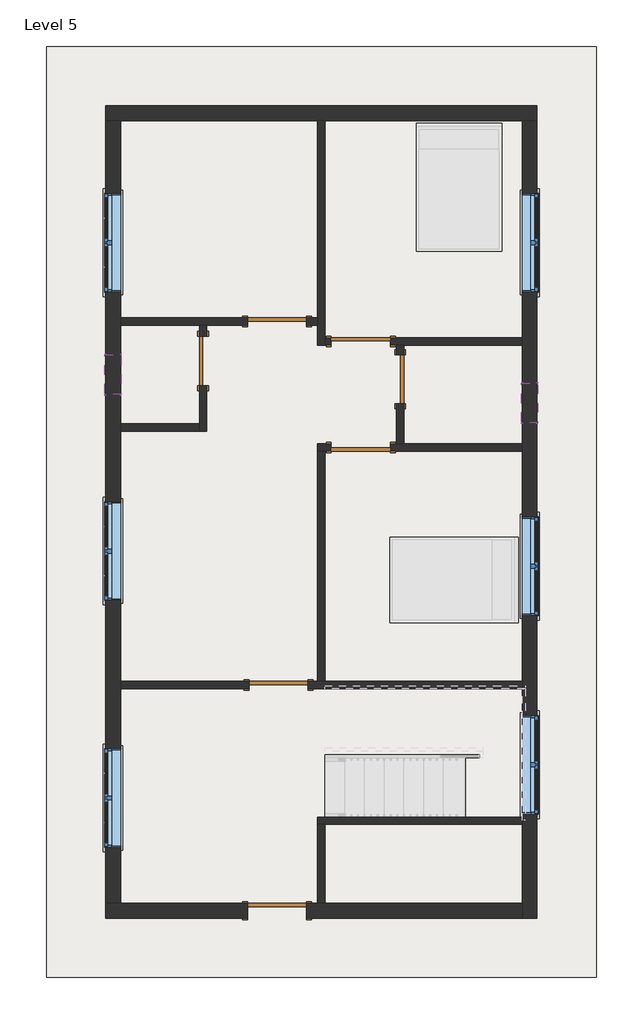
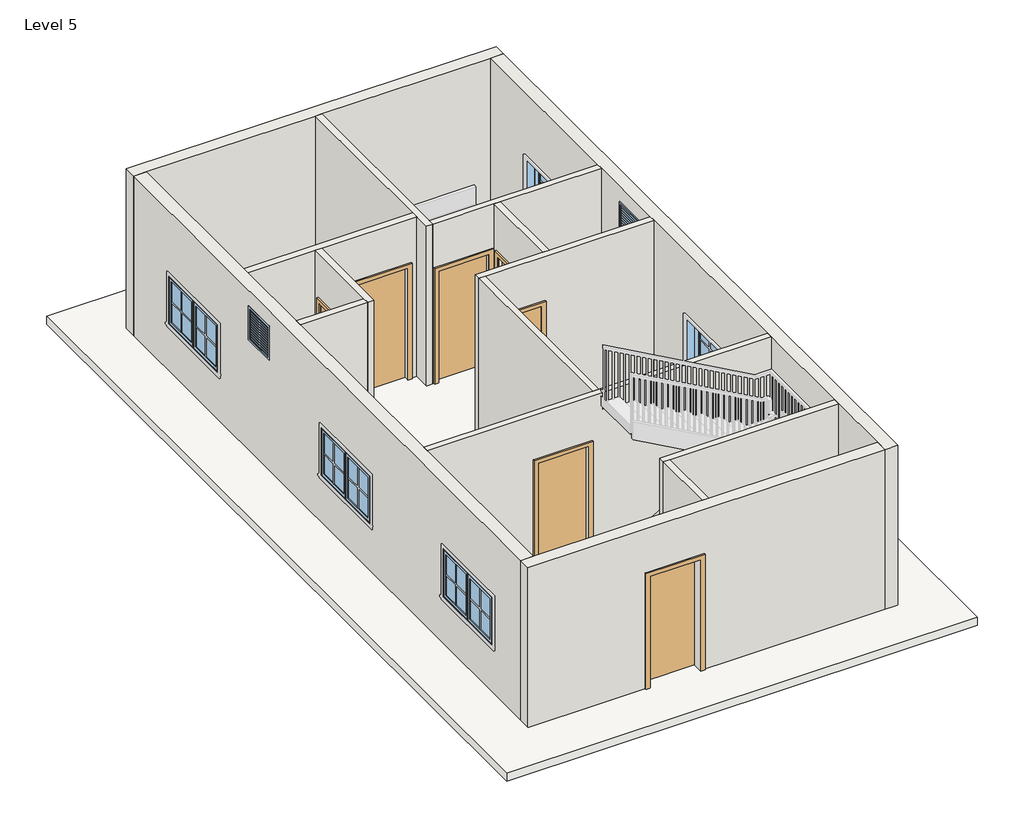
# One storey, part 1 of 3: 15 walls, 8 windows, 7 doors, 1 roof.
"""IFC4 building model written with IfcOpenShell, lengths in millimetres."""

from ifc_helpers import new_model, si_unit, frame, origin, place, context, project, spatial, polyline, outline, extrude, faceted_brep, transform, mapped, element, save
from components import door_78caadf7, door_214872d5, single_flush_door_3_e5f9f3c4, single_flush_door_3_305aa2a5, single_flush_door_3_0ca8825f, window_casement_double_win_5_c1d95f0f, window_f2d8fef0

model = new_model("IFC4")

# Units and contexts
model_context = context("Model", 3, world=origin())
ifc_project = project(units=[si_unit("LENGTHUNIT", "METRE", prefix="MILLI")], contexts=[model_context])

# Site, building, storey
site = spatial("IfcSite", under=ifc_project)
building = spatial("IfcBuilding", under=site)
storey = spatial("IfcBuildingStorey", under=building, Name="Level 5", Elevation=12649.2)

# Doors
placement = place(None, origin())
door_shape = door_78caadf7(model_context)
element("IfcDoor", 1, ObjectType="Single-Flush : 2'6\"", at=placement, inside=storey, context=model_context, shape_type="MappedRepresentation", body=[
    mapped(door_shape, transform((-35.92188, 1946.24131, 12649.2), x_axis=(0.0, 1.0, 0.0), y_axis=(-1.0, 0.0, 0.0), z_axis=(0.0, 0.0, 1.0))),
])
door_2_shape = door_214872d5(model_context)
element("IfcDoor", 2, ObjectType="Single-Flush : 2'6\"", at=placement, inside=storey, context=model_context, shape_type="MappedRepresentation", body=[
    mapped(door_2_shape, transform((-3083.92188, 2225.64131, 12649.2), x_axis=(0.0, 1.0, 0.0), y_axis=(-1.0, 0.0, 0.0), z_axis=(0.0, 0.0, 1.0))),
])
single_flush_door_3_shape = single_flush_door_3_e5f9f3c4(model_context)
element("IfcDoor", 3, ObjectType="Single-Flush : DOOR 3'", at=placement, inside=storey, context=model_context, shape_type="MappedRepresentation", body=[
    mapped(single_flush_door_3_shape, transform((-1940.92188, 2835.24131, 12649.2), x_axis=(1.0, 0.0, 0.0), y_axis=(0.0, 1.0, 0.0), z_axis=(0.0, 0.0, 1.0))),
])
element("IfcDoor", 4, ObjectType="Single-Flush : DOOR 3'", at=placement, inside=storey, context=model_context, shape_type="MappedRepresentation", body=[
    mapped(single_flush_door_3_shape, transform((-645.52188, 892.14131, 12649.2), x_axis=(-1.0, 0.0, 0.0), y_axis=(0.0, -1.0, 0.0), z_axis=(0.0, 0.0, 1.0))),
])
element("IfcDoor", 5, ObjectType="Single-Flush : DOOR 3'", at=placement, inside=storey, context=model_context, shape_type="MappedRepresentation", body=[
    mapped(single_flush_door_3_shape, transform((-1915.52188, -2778.15869, 12649.2), x_axis=(1.0, 0.0, 0.0), y_axis=(0.0, 1.0, 0.0), z_axis=(0.0, 0.0, 1.0))),
])
single_flush_door_3_2_shape = single_flush_door_3_305aa2a5(model_context)
element("IfcDoor", 6, ObjectType="Single-Flush : DOOR 3'", at=placement, inside=storey, context=model_context, shape_type="MappedRepresentation", body=[
    mapped(single_flush_door_3_2_shape, transform((-645.52188, 2530.44131, 12649.2), x_axis=(-1.0, 0.0, 0.0), y_axis=(0.0, -1.0, 0.0), z_axis=(0.0, 0.0, 1.0))),
])
single_flush_door_3_3_shape = single_flush_door_3_0ca8825f(model_context)
element("IfcDoor", 7, ObjectType="Single-Flush : DOOR 3'", at=placement, inside=storey, context=model_context, shape_type="MappedRepresentation", body=[
    mapped(single_flush_door_3_3_shape, transform((-1940.92188, -6264.30869, 12649.2), x_axis=(1.0, 0.0, 0.0), y_axis=(0.0, 1.0, 0.0), z_axis=(0.0, 0.0, 1.0))),
])

# Roof
element("IfcRoof", 8, ObjectType="ROOF 6\"", at=placement, inside=storey, context=model_context, shape_type="SweptSolid", body=[
    extrude(outline(polyline([(-5503.27188, 7083.39131), (2993.02812, 7083.39131), (2993.02812, -7293.00869), (-5503.27188, -7293.00869), (-5503.27188, 7083.39131)])), frame((0.0, 0.0, 12496.8), z_axis=(0.0, 0.0, 1.0), x_axis=(1.0, 0.0, 0.0)), (0.0, 0.0, 1.0), 152.4),
])

# Walls
element("IfcWall", 9, ObjectType="WALL 4.5'", at=placement, inside=storey, context=model_context, shape_type="Brep", body=[
    faceted_brep([(-1312.27188, 5940.39131, 12649.2), (-1312.27188, 2892.39131, 12649.2), (-1312.27188, 2778.09131, 12649.2), (-1312.27188, 2473.29131, 12649.2), (-1312.27188, 2473.29131, 15697.2), (-1312.27188, 2778.09131, 15697.2), (-1312.27188, 2892.39131, 15697.2), (-1312.27188, 5940.39131, 15697.2), (-1197.97188, 5940.39131, 12649.2), (-1197.97188, 5940.39131, 15697.2), (-1197.97188, 2587.59131, 15697.2), (-1197.97188, 2473.29131, 15697.2), (-1197.97188, 2473.29131, 12649.2), (-1197.97188, 2587.59131, 12649.2)], [[[0, 1, 2, 3, 4, 5, 6, 7]], [[8, 9, 10, 11, 12, 13]], [[3, 2, 1, 0, 8, 13, 12]], [[0, 7, 9, 8]], [[4, 3, 12, 11]], [[7, 6, 5, 4, 11, 10, 9]]]),
])
element("IfcWall", 10, ObjectType="WALL 4.5'", at=placement, inside=storey, context=model_context, shape_type="Brep", body=[
    faceted_brep([(-1197.97188, 2473.29131, 12649.2), (-1102.72188, 2473.29131, 12649.2), (-1102.72188, 2473.29131, 14782.8), (-188.32188, 2473.29131, 14782.8), (-188.32188, 2473.29131, 12649.2), (-93.07188, 2473.29131, 12649.2), (21.22812, 2473.29131, 12649.2), (1850.02812, 2473.29131, 12649.2), (1850.02812, 2473.29131, 15697.2), (21.22812, 2473.29131, 15697.2), (-93.07188, 2473.29131, 15697.2), (-1197.97188, 2473.29131, 15697.2), (-1102.72188, 2587.59131, 14782.8), (-1102.72188, 2587.59131, 12649.2), (-1197.97188, 2587.59131, 12649.2), (-1197.97188, 2587.59131, 15697.2), (1850.02812, 2587.59131, 15697.2), (1850.02812, 2587.59131, 12649.2), (-188.32188, 2587.59131, 12649.2), (-188.32188, 2587.59131, 14782.8)], [[[0, 1, 2, 3, 4, 5, 6, 7, 8, 9, 10, 11]], [[12, 13, 14, 15, 16, 17, 18, 19]], [[18, 17, 7, 6, 5, 4]], [[14, 13, 1, 0]], [[0, 11, 15, 14]], [[8, 7, 17, 16]], [[2, 1, 13, 12]], [[3, 2, 12, 19]], [[4, 3, 19, 18]], [[11, 10, 9, 8, 16, 15]]]),
])
element("IfcWall", 11, ObjectType="WALL 4.5'", at=placement, inside=storey, context=model_context, shape_type="Brep", body=[
    faceted_brep([(-1312.27188, 2892.39131, 12649.2), (-1483.72188, 2892.39131, 12649.2), (-1483.72188, 2892.39131, 14782.8), (-2398.12188, 2892.39131, 14782.8), (-2398.12188, 2892.39131, 12649.2), (-4360.27188, 2892.39131, 12649.2), (-4360.27188, 2892.39131, 15697.2), (-1312.27188, 2892.39131, 15697.2), (-1483.72188, 2778.09131, 14782.8), (-1483.72188, 2778.09131, 12649.2), (-1312.27188, 2778.09131, 12649.2), (-1312.27188, 2778.09131, 15697.2), (-3026.77188, 2778.09131, 15697.2), (-3141.07188, 2778.09131, 15697.2), (-4360.27188, 2778.09131, 15697.2), (-4360.27188, 2778.09131, 12649.2), (-3141.07188, 2778.09131, 12649.2), (-3026.77188, 2778.09131, 12649.2), (-2398.12188, 2778.09131, 12649.2), (-2398.12188, 2778.09131, 14782.8)], [[[0, 1, 2, 3, 4, 5, 6, 7]], [[8, 9, 10, 11, 12, 13, 14, 15, 16, 17, 18, 19]], [[10, 9, 1, 0]], [[18, 17, 16, 15, 5, 4]], [[6, 5, 15, 14]], [[0, 7, 11, 10]], [[2, 1, 9, 8]], [[3, 2, 8, 19]], [[4, 3, 19, 18]], [[7, 6, 14, 13, 12, 11]]]),
])
element("IfcWall", 12, ObjectType="WALL 4.5'", at=placement, inside=storey, context=model_context, shape_type="Brep", body=[
    faceted_brep([(-3141.07188, 2778.09131, 12649.2), (-3141.07188, 2606.64131, 12649.2), (-3141.07188, 2606.64131, 14782.8), (-3141.07188, 1844.64131, 14782.8), (-3141.07188, 1844.64131, 12649.2), (-3141.07188, 1254.09131, 12649.2), (-3141.07188, 1139.79131, 12649.2), (-3141.07188, 1139.79131, 15697.2), (-3141.07188, 1254.09131, 15697.2), (-3141.07188, 2778.09131, 15697.2), (-3026.77188, 2606.64131, 14782.8), (-3026.77188, 2606.64131, 12649.2), (-3026.77188, 2778.09131, 12649.2), (-3026.77188, 2778.09131, 15697.2), (-3026.77188, 1139.79131, 15697.2), (-3026.77188, 1139.79131, 12649.2), (-3026.77188, 1844.64131, 12649.2), (-3026.77188, 1844.64131, 14782.8)], [[[0, 1, 2, 3, 4, 5, 6, 7, 8, 9]], [[10, 11, 12, 13, 14, 15, 16, 17]], [[16, 15, 6, 5, 4]], [[12, 11, 1, 0]], [[0, 9, 13, 12]], [[7, 6, 15, 14]], [[2, 1, 11, 10]], [[3, 2, 10, 17]], [[4, 3, 17, 16]], [[9, 8, 7, 14, 13]]]),
])
element("IfcWall", 13, ObjectType="WALL 4.5'", at=placement, inside=storey, context=model_context, shape_type="SweptSolid", body=[
    extrude(outline(polyline([(-4360.27188, 1254.09131), (-3141.07188, 1254.09131), (-3141.07188, 1139.79131), (-4360.27188, 1139.79131), (-4360.27188, 1254.09131)])), frame((0.0, 0.0, 12649.2), z_axis=(0.0, 0.0, 1.0), x_axis=(1.0, 0.0, 0.0)), (0.0, 0.0, 1.0), 3048.0),
])
element("IfcWall", 14, ObjectType="WALL 4.5'", at=placement, inside=storey, context=model_context, shape_type="SweptSolid", body=[
    extrude(outline(polyline([(2473.29131, 12649.2), (2327.24131, 12649.2), (2327.24131, 14782.8), (1565.24131, 14782.8), (1565.24131, 12649.2), (949.29131, 12649.2), (949.29131, 15697.2), (2473.29131, 15697.2), (2473.29131, 12649.2)])), frame((-93.07188, 0.0, 0.0), z_axis=(1.0, 0.0, 0.0), x_axis=(0.0, 1.0, 0.0)), (0.0, 0.0, 1.0), 114.3),
])
element("IfcWall", 15, ObjectType="WALL 4.5'", at=placement, inside=storey, context=model_context, shape_type="Brep", body=[
    faceted_brep([(-1102.72188, 949.29131, 14782.8), (-1102.72188, 949.29131, 12649.2), (-1312.27188, 949.29131, 12649.2), (-1312.27188, 949.29131, 15697.2), (-93.07188, 949.29131, 15697.2), (21.22812, 949.29131, 15697.2), (1850.02812, 949.29131, 15697.2), (1850.02812, 949.29131, 12649.2), (21.22812, 949.29131, 12649.2), (-93.07188, 949.29131, 12649.2), (-188.32188, 949.29131, 12649.2), (-188.32188, 949.29131, 14782.8), (-1312.27188, 834.99131, 12649.2), (-1197.97188, 834.99131, 12649.2), (-1102.72188, 834.99131, 12649.2), (-1102.72188, 834.99131, 14782.8), (-188.32188, 834.99131, 14782.8), (-188.32188, 834.99131, 12649.2), (1850.02812, 834.99131, 12649.2), (1850.02812, 834.99131, 15697.2), (-1197.97188, 834.99131, 15697.2), (-1312.27188, 834.99131, 15697.2)], [[[0, 1, 2, 3, 4, 5, 6, 7, 8, 9, 10, 11]], [[12, 13, 14, 15, 16, 17, 18, 19, 20, 21]], [[2, 1, 14, 13, 12]], [[10, 9, 8, 7, 18, 17]], [[7, 6, 19, 18]], [[3, 2, 12, 21]], [[15, 14, 1, 0]], [[16, 15, 0, 11]], [[17, 16, 11, 10]], [[6, 5, 4, 3, 21, 20, 19]]]),
])
element("IfcWall", 16, ObjectType="WALL 4.5'", at=placement, inside=storey, context=model_context, shape_type="SweptSolid", body=[
    extrude(outline(polyline([(-1312.27188, -2721.00869), (-1312.27188, 834.99131), (-1197.97188, 834.99131), (-1197.97188, -2721.00869), (-1312.27188, -2721.00869)])), frame((0.0, 0.0, 12649.2), z_axis=(0.0, 0.0, 1.0), x_axis=(1.0, 0.0, 0.0)), (0.0, 0.0, 1.0), 3048.0),
])
element("IfcWall", 17, ObjectType="WALL 4.5'", at=placement, inside=storey, context=model_context, shape_type="Brep", body=[
    faceted_brep([(1850.02812, -2721.00869, 12649.2), (-1197.97188, -2721.00869, 12649.2), (-1312.27188, -2721.00869, 12649.2), (-1458.32188, -2721.00869, 12649.2), (-1458.32188, -2721.00869, 14782.8), (-2372.72188, -2721.00869, 14782.8), (-2372.72188, -2721.00869, 12649.2), (-4360.27188, -2721.00869, 12649.2), (-4360.27188, -2721.00869, 15697.2), (-1312.27188, -2721.00869, 15697.2), (-1197.97188, -2721.00869, 15697.2), (1850.02812, -2721.00869, 15697.2), (-1458.32188, -2835.30869, 14782.8), (-1458.32188, -2835.30869, 12649.2), (1850.02812, -2835.30869, 12649.2), (1850.02812, -2835.30869, 15697.2), (-4360.27188, -2835.30869, 15697.2), (-4360.27188, -2835.30869, 12649.2), (-2372.72188, -2835.30869, 12649.2), (-2372.72188, -2835.30869, 14782.8)], [[[0, 1, 2, 3, 4, 5, 6, 7, 8, 9, 10, 11]], [[12, 13, 14, 15, 16, 17, 18, 19]], [[18, 17, 7, 6]], [[14, 13, 3, 2, 1, 0]], [[0, 11, 15, 14]], [[8, 7, 17, 16]], [[4, 3, 13, 12]], [[5, 4, 12, 19]], [[6, 5, 19, 18]], [[11, 10, 9, 8, 16, 15]]]),
])
element("IfcWall", 18, ObjectType="WALL 4.5'", at=placement, inside=storey, context=model_context, shape_type="Brep", body=[
    faceted_brep([(1850.02812, -4816.50869, 12649.2), (-1312.27188, -4816.50869, 12649.2), (-1312.27188, -4816.50869, 15697.2), (1850.02812, -4816.50869, 15697.2), (1850.02812, -4930.80869, 12649.2), (1850.02812, -4930.80869, 15697.2), (-1197.97188, -4930.80869, 15697.2), (-1312.27188, -4930.80869, 15697.2), (-1312.27188, -4930.80869, 12649.2), (-1197.97188, -4930.80869, 12649.2)], [[[0, 1, 2, 3]], [[4, 5, 6, 7, 8, 9]], [[1, 0, 4, 9, 8]], [[0, 3, 5, 4]], [[2, 1, 8, 7]], [[3, 2, 7, 6, 5]]]),
])
element("IfcWall", 19, ObjectType="WALL 4.5'", at=placement, inside=storey, context=model_context, shape_type="SweptSolid", body=[
    extrude(outline(polyline([(-1312.27188, -6150.00869), (-1312.27188, -4930.80869), (-1197.97188, -4930.80869), (-1197.97188, -6150.00869), (-1312.27188, -6150.00869)])), frame((0.0, 0.0, 12649.2), z_axis=(0.0, 0.0, 1.0), x_axis=(1.0, 0.0, 0.0)), (0.0, 0.0, 1.0), 3048.0),
])
element("IfcWall", 20, ObjectType="WALL 9\"", at=placement, inside=storey, context=model_context, shape_type="Brep", body=[
    faceted_brep([(-4588.87188, 5940.39131, 12649.2), (-4360.27188, 5940.39131, 12649.2), (-1312.27188, 5940.39131, 12649.2), (-1197.97188, 5940.39131, 12649.2), (1850.02812, 5940.39131, 12649.2), (2078.62812, 5940.39131, 12649.2), (2078.62812, 5940.39131, 15697.2), (1850.02812, 5940.39131, 15697.2), (-1197.97188, 5940.39131, 15697.2), (-1312.27188, 5940.39131, 15697.2), (-4360.27188, 5940.39131, 15697.2), (-4588.87188, 5940.39131, 15697.2), (-4588.87188, 6168.99131, 12649.2), (-4588.87188, 6168.99131, 15697.2), (2078.62812, 6168.99131, 15697.2), (2078.62812, 6168.99131, 12649.2)], [[[0, 1, 2, 3, 4, 5, 6, 7, 8, 9, 10, 11]], [[12, 13, 14, 15]], [[5, 4, 3, 2, 1, 0, 12, 15]], [[6, 5, 15, 14]], [[0, 11, 13, 12]], [[11, 10, 9, 8, 7, 6, 14, 13]]]),
])
element("IfcWall", 21, ObjectType="WALL 9\"", at=placement, inside=storey, context=model_context, shape_type="Brep", body=[
    faceted_brep([(1850.02812, 5940.39131, 12649.2), (1850.02812, 2587.59131, 12649.2), (1850.02812, 2473.29131, 12649.2), (1850.02812, 949.29131, 12649.2), (1850.02812, 834.99131, 12649.2), (1850.02812, -2721.00869, 12649.2), (1850.02812, -2835.30869, 12649.2), (1850.02812, -4816.50869, 12649.2), (1850.02812, -4930.80869, 12649.2), (1850.02812, -6150.00869, 12649.2), (1850.02812, -6378.60869, 12649.2), (1850.02812, -6378.60869, 15697.2), (1850.02812, -6150.00869, 15697.2), (1850.02812, -4930.80869, 15697.2), (1850.02812, -4816.50869, 15697.2), (1850.02812, -2835.30869, 15697.2), (1850.02812, -2721.00869, 15697.2), (1850.02812, 834.99131, 15697.2), (1850.02812, 949.29131, 15697.2), (1850.02812, 2473.29131, 15697.2), (1850.02812, 2587.59131, 15697.2), (1850.02812, 5940.39131, 15697.2), (1850.02812, -4772.05869, 14478.0), (1850.02812, -4772.05869, 13563.6), (1850.02812, -3248.05869, 13563.6), (1850.02812, -3248.05869, 14478.0), (1850.02812, 3292.44131, 14478.0), (1850.02812, 3292.44131, 13563.6), (1850.02812, 4816.44131, 13563.6), (1850.02812, 4816.44131, 14478.0), (1850.02812, -1705.00869, 14478.0), (1850.02812, -1705.00869, 13563.6), (1850.02812, -181.00869, 13563.6), (1850.02812, -181.00869, 14478.0), (1850.02812, 1273.14131, 15392.4), (1850.02812, 1273.14131, 14782.8), (1850.02812, 1882.74131, 14782.8), (1850.02812, 1882.74131, 15392.4), (2078.62812, 5940.39131, 12649.2), (2078.62812, 5940.39131, 15697.2), (2078.62812, -6378.60869, 15697.2), (2078.62812, -6378.60869, 12649.2), (2078.62812, -4772.05869, 14478.0), (2078.62812, -3248.05869, 14478.0), (2078.62812, -3248.05869, 13563.6), (2078.62812, -4772.05869, 13563.6), (2078.62812, 3292.44131, 14478.0), (2078.62812, 4816.44131, 14478.0), (2078.62812, 4816.44131, 13563.6), (2078.62812, 3292.44131, 13563.6), (2078.62812, -1705.00869, 14478.0), (2078.62812, -181.00869, 14478.0), (2078.62812, -181.00869, 13563.6), (2078.62812, -1705.00869, 13563.6), (2078.62812, 1273.14131, 15392.4), (2078.62812, 1882.74131, 15392.4), (2078.62812, 1882.74131, 14782.8), (2078.62812, 1273.14131, 14782.8)], [[[0, 1, 2, 3, 4, 5, 6, 7, 8, 9, 10, 11, 12, 13, 14, 15, 16, 17, 18, 19, 20, 21], [22, 23, 24, 25], [26, 27, 28, 29], [30, 31, 32, 33], [34, 35, 36, 37]], [[38, 39, 40, 41], [42, 43, 44, 45], [46, 47, 48, 49], [50, 51, 52, 53], [54, 55, 56, 57]], [[10, 9, 8, 7, 6, 5, 4, 3, 2, 1, 0, 38, 41]], [[0, 21, 39, 38]], [[11, 10, 41, 40]], [[23, 22, 42, 45]], [[24, 23, 45, 44]], [[25, 24, 44, 43]], [[22, 25, 43, 42]], [[27, 26, 46, 49]], [[28, 27, 49, 48]], [[29, 28, 48, 47]], [[26, 29, 47, 46]], [[31, 30, 50, 53]], [[32, 31, 53, 52]], [[33, 32, 52, 51]], [[30, 33, 51, 50]], [[35, 34, 54, 57]], [[36, 35, 57, 56]], [[37, 36, 56, 55]], [[34, 37, 55, 54]], [[21, 20, 19, 18, 17, 16, 15, 14, 13, 12, 11, 40, 39]]]),
])
element("IfcWall", 22, ObjectType="WALL 9\"", at=placement, inside=storey, context=model_context, shape_type="Brep", body=[
    faceted_brep([(1850.02812, -6150.00869, 12649.2), (-1197.97188, -6150.00869, 12649.2), (-1312.27188, -6150.00869, 12649.2), (-1483.72188, -6150.00869, 12649.2), (-1483.72188, -6150.00869, 14782.8), (-2398.12188, -6150.00869, 14782.8), (-2398.12188, -6150.00869, 12649.2), (-4360.27188, -6150.00869, 12649.2), (-4588.87188, -6150.00869, 12649.2), (-4588.87188, -6150.00869, 15697.2), (-4360.27188, -6150.00869, 15697.2), (-1312.27188, -6150.00869, 15697.2), (-1197.97188, -6150.00869, 15697.2), (1850.02812, -6150.00869, 15697.2), (-1483.72188, -6378.60869, 14782.8), (-1483.72188, -6378.60869, 12649.2), (1850.02812, -6378.60869, 12649.2), (1850.02812, -6378.60869, 15697.2), (-4588.87188, -6378.60869, 15697.2), (-4588.87188, -6378.60869, 12649.2), (-2398.12188, -6378.60869, 12649.2), (-2398.12188, -6378.60869, 14782.8)], [[[0, 1, 2, 3, 4, 5, 6, 7, 8, 9, 10, 11, 12, 13]], [[14, 15, 16, 17, 18, 19, 20, 21]], [[20, 19, 8, 7, 6]], [[16, 15, 3, 2, 1, 0]], [[0, 13, 17, 16]], [[9, 8, 19, 18]], [[4, 3, 15, 14]], [[5, 4, 14, 21]], [[6, 5, 21, 20]], [[13, 12, 11, 10, 9, 18, 17]]]),
])
element("IfcWall", 23, ObjectType="WALL 9\"", at=placement, inside=storey, context=model_context, shape_type="Brep", body=[
    faceted_brep([(-4360.27188, -6150.00869, 12649.2), (-4360.27188, -2835.30869, 12649.2), (-4360.27188, -2721.00869, 12649.2), (-4360.27188, 1139.79131, 12649.2), (-4360.27188, 1254.09131, 12649.2), (-4360.27188, 2778.09131, 12649.2), (-4360.27188, 2892.39131, 12649.2), (-4360.27188, 5940.39131, 12649.2), (-4360.27188, 5940.39131, 15697.2), (-4360.27188, 2892.39131, 15697.2), (-4360.27188, 2778.09131, 15697.2), (-4360.27188, 1254.09131, 15697.2), (-4360.27188, 1139.79131, 15697.2), (-4360.27188, -2721.00869, 15697.2), (-4360.27188, -2835.30869, 15697.2), (-4360.27188, -6150.00869, 15697.2), (-4360.27188, 4816.44131, 14478.0), (-4360.27188, 4816.44131, 13563.6), (-4360.27188, 3292.44131, 13563.6), (-4360.27188, 3292.44131, 14478.0), (-4360.27188, 53.94131, 14478.0), (-4360.27188, 53.94131, 13563.6), (-4360.27188, -1470.05869, 13563.6), (-4360.27188, -1470.05869, 14478.0), (-4360.27188, -3759.23369, 14478.0), (-4360.27188, -3759.23369, 13563.6), (-4360.27188, -5283.23369, 13563.6), (-4360.27188, -5283.23369, 14478.0), (-4360.27188, 1711.29131, 15392.4), (-4360.27188, 2320.89131, 15392.4), (-4360.27188, 2320.89131, 14782.8), (-4360.27188, 1711.29131, 14782.8), (-4588.87188, -6150.00869, 12649.2), (-4588.87188, -6150.00869, 15697.2), (-4588.87188, 5940.39131, 15697.2), (-4588.87188, 5940.39131, 12649.2), (-4588.87188, 4816.44131, 14478.0), (-4588.87188, 3292.44131, 14478.0), (-4588.87188, 3292.44131, 13563.6), (-4588.87188, 4816.44131, 13563.6), (-4588.87188, 53.94131, 14478.0), (-4588.87188, -1470.05869, 14478.0), (-4588.87188, -1470.05869, 13563.6), (-4588.87188, 53.94131, 13563.6), (-4588.87188, -3759.23369, 14478.0), (-4588.87188, -5283.23369, 14478.0), (-4588.87188, -5283.23369, 13563.6), (-4588.87188, -3759.23369, 13563.6), (-4588.87188, 1711.29131, 15392.4), (-4588.87188, 1711.29131, 14782.8), (-4588.87188, 2320.89131, 14782.8), (-4588.87188, 2320.89131, 15392.4)], [[[0, 1, 2, 3, 4, 5, 6, 7, 8, 9, 10, 11, 12, 13, 14, 15], [16, 17, 18, 19], [20, 21, 22, 23], [24, 25, 26, 27], [28, 29, 30, 31]], [[32, 33, 34, 35], [36, 37, 38, 39], [40, 41, 42, 43], [44, 45, 46, 47], [48, 49, 50, 51]], [[7, 6, 5, 4, 3, 2, 1, 0, 32, 35]], [[8, 7, 35, 34]], [[0, 15, 33, 32]], [[17, 16, 36, 39]], [[18, 17, 39, 38]], [[19, 18, 38, 37]], [[16, 19, 37, 36]], [[21, 20, 40, 43]], [[22, 21, 43, 42]], [[23, 22, 42, 41]], [[20, 23, 41, 40]], [[25, 24, 44, 47]], [[26, 25, 47, 46]], [[27, 26, 46, 45]], [[24, 27, 45, 44]], [[49, 48, 28, 31]], [[50, 49, 31, 30]], [[51, 50, 30, 29]], [[48, 51, 29, 28]], [[15, 14, 13, 12, 11, 10, 9, 8, 34, 33]]]),
])

# Windows
window_casement_double_win_5_shape = window_casement_double_win_5_c1d95f0f(model_context)
element("IfcWindow", 24, ObjectType="Window-Casement-Double : WIN 5'", at=placement, inside=storey, context=model_context, shape_type="MappedRepresentation", body=[
    mapped(window_casement_double_win_5_shape, transform((-4474.57188, 4054.44131, 12649.2), x_axis=(0.0, 1.0, 0.0), y_axis=(-1.0, 0.0, 0.0), z_axis=(0.0, 0.0, 1.0))),
])
element("IfcWindow", 25, ObjectType="Window-Casement-Double : WIN 5'", at=placement, inside=storey, context=model_context, shape_type="MappedRepresentation", body=[
    mapped(window_casement_double_win_5_shape, transform((-4474.57188, -708.05869, 12649.2), x_axis=(0.0, 1.0, 0.0), y_axis=(-1.0, 0.0, 0.0), z_axis=(0.0, 0.0, 1.0))),
])
element("IfcWindow", 26, ObjectType="Window-Casement-Double : WIN 5'", at=placement, inside=storey, context=model_context, shape_type="MappedRepresentation", body=[
    mapped(window_casement_double_win_5_shape, transform((-4474.57188, -4521.23369, 12649.2), x_axis=(0.0, 1.0, 0.0), y_axis=(-1.0, 0.0, 0.0), z_axis=(0.0, 0.0, 1.0))),
])
element("IfcWindow", 27, ObjectType="Window-Casement-Double : WIN 5'", at=placement, inside=storey, context=model_context, shape_type="MappedRepresentation", body=[
    mapped(window_casement_double_win_5_shape, transform((1964.32812, -4010.05869, 12649.2), x_axis=(0.0, -1.0, 0.0), y_axis=(1.0, 0.0, 0.0), z_axis=(0.0, 0.0, 1.0))),
])
element("IfcWindow", 28, ObjectType="Window-Casement-Double : WIN 5'", at=placement, inside=storey, context=model_context, shape_type="MappedRepresentation", body=[
    mapped(window_casement_double_win_5_shape, transform((1964.32812, 4054.44131, 12649.2), x_axis=(0.0, -1.0, 0.0), y_axis=(1.0, 0.0, 0.0), z_axis=(0.0, 0.0, 1.0))),
])
element("IfcWindow", 29, ObjectType="Window-Casement-Double : WIN 5'", at=placement, inside=storey, context=model_context, shape_type="MappedRepresentation", body=[
    mapped(window_casement_double_win_5_shape, transform((1964.32812, -943.00869, 12649.2), x_axis=(0.0, -1.0, 0.0), y_axis=(1.0, 0.0, 0.0), z_axis=(0.0, 0.0, 1.0))),
])
window_shape = window_f2d8fef0(model_context)
element("IfcWindow", 30, ObjectType="Window-Louvers : 24\" x 24\"", at=placement, inside=storey, context=model_context, shape_type="MappedRepresentation", body=[
    mapped(window_shape, transform((1957.97812, 1577.94131, 13868.4), x_axis=(0.0, 1.0, 0.0), y_axis=(-1.0, 0.0, 0.0), z_axis=(0.0, 0.0, 1.0))),
])
element("IfcWindow", 31, ObjectType="Window-Louvers : 24\" x 24\"", at=placement, inside=storey, context=model_context, shape_type="MappedRepresentation", body=[
    mapped(window_shape, transform((-4480.92188, 2016.09131, 13868.4), x_axis=(0.0, 1.0, 0.0), y_axis=(-1.0, 0.0, 0.0), z_axis=(0.0, 0.0, 1.0))),
])

save(model, "model.ifc")

# Revit data of these elements
# Type "Single-Flush : 2'6\""
#   Type Mark = "9"
#   Construction Type Id = "MDOOR"
#   Assembly Code = "C1020"
#   Analytic Construction = "Metal"
#   Thickness = 0' - 2"
#   Heat Transfer Coefficient (U) = 0.651978 BTU/(h·ft²·°F)
#   Height = 7' - 0"
#   Trim Projection Ext = 0' - 1"
#   Trim Projection Int = 0' - 1"
#   Trim Width = 0' - 3"
#   Width = 2' - 6"
#   Define Thermal Properties by = 1
#   Door Material = Door - Panel
#   Frame Material = Door - Frame
#   Visual Light Transmittance = 0
#   Solar Heat Gain Coefficient = 0
#   Function = (empty or 0)
#   Wall Closure = (empty or 0)
# Type "Single-Flush : DOOR 3'"
#   Type Mark = "8"
#   Construction Type Id = "MDOOR"
#   Assembly Code = "C1020"
#   Analytic Construction = "Metal"
#   Thickness = 0' - 2"
#   Heat Transfer Coefficient (U) = 0.651978 BTU/(h·ft²·°F)
#   Height = 7' - 0"
#   Trim Projection Ext = 0' - 1"
#   Trim Projection Int = 0' - 1"
#   Trim Width = 0' - 3"
#   Width = 3' - 0"
#   Define Thermal Properties by = 1
#   Door Material = Door - Panel
#   Frame Material = Door - Frame
#   Visual Light Transmittance = 0
#   Solar Heat Gain Coefficient = 0
#   Function = (empty or 0)
#   Wall Closure = (empty or 0)
# Type "ROOF 6\""
#   Assembly Code = "B1020"
#   Layers, outside or top first: 0' - 6" no material (function 1)
# Type "WALL 4.5'"
#   Assembly Code = "B2010"
#   Layers, outside or top first: 0' - 4 1/2" no material (function 1)
# Type "WALL 9\""
#   Assembly Code = "B2010"
#   Layers, outside or top first: 0' - 9" no material (function 1)
# Type "Window-Casement-Double : WIN 5'"
#   Type Mark = "18"
#   Fire Rating = "0.5h"
#   Assembly Code = "B2020100"
#   Analytic Construction = "Double glazing - domestic"
#   Frame Extension [instance default] = 0' - 0 1/4"
#   Window Inset [instance default] = 0' - 0"
#   Wall Thickness [instance default] = 0' - 6"
#   Interior Wall Closure [instance default] = 0' - 2 1/4"
#   Half Width = 2' - 6"
#   Visual Light Transmittance = 0.81
#   Thermal Resistance (R) = 1.8146 (h·ft²·°F)/BTU
#   Solar Heat Gain Coefficient = 0.76
#   Rough Width = 5' - 0 1/2"
#   Rough Height = 3' - 0 1/2"
#   Height = 3' - 0"
#   Heat Transfer Coefficient (U) = 0.5511 BTU/(h·ft²·°F)
#   Exterior Wall Closure [instance default] = 0' - 1 1/4"
#   Extension Jamb [instance default] = 0' - 2 1/4"
#   Default Sill Height = 3' - 0"
#   Width = 5' - 0"
#   Muntin Visibility = yes
#   Interior Trim Visibility [instance default] = yes
#   Exterior Trim Visibility [instance default] = yes
#   Extension Jamb Visibility [instance default] = yes
#   Interior Trim Material = Wood - Stained
#   Muntin Pattern = Muntin Pattern_2x2 : Muntin Pattern_2x2
#   Interior Trim = Trim-Window-Interior-Flat : Picture Frame
#   Interior Frame Material = Wood - Stained
#   Glass Panel Material = Glass
#   Exterior Trim Material = Clad - White
#   Exterior Trim = Trim-Window-Exterior-Flat : with Sill
#   Exterior Frame Material = Clad - White
#   Wall Closure = (empty or 0)
# Type "Window-Louvers : 24\" x 24\""
#   Type Mark = "19"
#   Construction Type Id = "GSP4R"
#   Assembly Code = "B20"
#   Analytic Construction = "1/8 in Pilkington single glazing"
#   Visual Light Transmittance = 0.9
#   Thermal Resistance (R) = 1.53941 (h·ft²·°F)/BTU
#   Solar Heat Gain Coefficient = 0.78
#   Max Height = 1' - 11.74264"
#   Height = 2' - 0"
#   Heat Transfer Coefficient (U) = 0.6496 BTU/(h·ft²·°F)
#   Blade Width [instance default] = 1' - 10 1/2"
#   Blade Vertical Thickness = 0' - 0.35355"
#   Blade Thickness = 0' - 0 1/4"
#   Blade Spacing = 0' - 1 1/2"
#   Blade Height = 0' - 1.85355"
#   Blade Depth = 0' - 3"
#   Blade Angle = 45.00°
#   Default Sill Height = 3' - 0"
#   Trim Projection_Exterior = 0' - 0 1/2"
#   Trim Projection_Interior = 0' - 0 1/2"
#   Trim Width_Exterior = 0' - 1 1/2"
#   Trim Width_Interior = 0' - 1 1/2"
#   Width = 2' - 0"
#   Max Blade Count = 12
#   Define Thermal Properties by = 1
#   Blade Count = 12
#   Frame Material = Birch
#   Louver Material = Birch
#   Trim Exterior Material = Birch
#   Trim Interior Material = Birch
#   Wall Closure = (empty or 0)
# Elements 1, 2 (IfcDoor, "Single-Flush : 2'6\"")
#   Phase Created = New Construction
#   Materials on its faces: "Door - Frame", "Door - Panel"
# Elements 3, 4, 5, 6, 7 (IfcDoor, "Single-Flush : DOOR 3'")
#   Phase Created = New Construction
#   Materials on its faces: "Door - Frame", "Door - Panel"
# Element 8 (IfcRoof, "ROOF 6\"")
#   built-in parameter 1001705 = 41.5 (stored number, unit not read)
#   built-in parameter 1001701 = -0.5 (stored number, unit not read)
#   built-in parameter 1001710 = 33615
#   Phase Created = New Construction
#   Materials on its faces: "Parking Stripe", "Default Roof", "Wood - Stained"
# Elements 9, 10, 11, 12, 13, 14, 15, 16, 17, 18, 19 (IfcWall, "WALL 4.5'")
#   Top Offset = 0' - 0"
#   Base Offset = 0' - 0"
#   Unconnected Height = 10' - 0"
#   wall height = 10' - 0"
#   Phase Created = New Construction
#   Base Constraint = Level 5
#   Materials on its faces: "Default Wall"
# Elements 20, 21, 22, 23 (IfcWall, "WALL 9\"")
#   Top Offset = 0' - 0"
#   Base Offset = 0' - 0"
#   Unconnected Height = 10' - 0"
#   wall height = 10' - 0"
#   Phase Created = New Construction
#   Base Constraint = Level 5
#   Materials on its faces: "Default Wall", "Copper"
# Element 24 (IfcWindow, "Window-Casement-Double : WIN 5'")
#   Mark = "33"
#   Window Inset = 0' - 0"
#   Interior Wall Closure = 0' - 2 1/4"
#   Frame Extension = 0' - 0 1/4"
#   Exterior Wall Closure = 0' - 1 1/4"
#   Interior Trim Visibility = yes
#   Exterior Trim Visibility = yes
#   Phase Created = New Construction
#   Materials on its faces: "Wood - Stained", "Glass", "Clad - White"
# Element 25 (IfcWindow, "Window-Casement-Double : WIN 5'")
#   Mark = "34"
#   Window Inset = 0' - 0"
#   Interior Wall Closure = 0' - 2 1/4"
#   Frame Extension = 0' - 0 1/4"
#   Exterior Wall Closure = 0' - 1 1/4"
#   Interior Trim Visibility = yes
#   Exterior Trim Visibility = yes
#   Phase Created = New Construction
#   Materials on its faces: "Wood - Stained", "Glass", "Clad - White"
# Element 26 (IfcWindow, "Window-Casement-Double : WIN 5'")
#   Mark = "35"
#   Window Inset = 0' - 0"
#   Interior Wall Closure = 0' - 2 1/4"
#   Frame Extension = 0' - 0 1/4"
#   Exterior Wall Closure = 0' - 1 1/4"
#   Interior Trim Visibility = yes
#   Exterior Trim Visibility = yes
#   Phase Created = New Construction
#   Materials on its faces: "Wood - Stained", "Glass", "Clad - White"
# Element 27 (IfcWindow, "Window-Casement-Double : WIN 5'")
#   Mark = "36"
#   Window Inset = 0' - 0"
#   Interior Wall Closure = 0' - 2 1/4"
#   Frame Extension = 0' - 0 1/4"
#   Exterior Wall Closure = 0' - 1 1/4"
#   Interior Trim Visibility = yes
#   Exterior Trim Visibility = yes
#   Phase Created = New Construction
#   Materials on its faces: "Wood - Stained", "Glass", "Clad - White"
# Element 28 (IfcWindow, "Window-Casement-Double : WIN 5'")
#   Mark = "37"
#   Window Inset = 0' - 0"
#   Interior Wall Closure = 0' - 2 1/4"
#   Frame Extension = 0' - 0 1/4"
#   Exterior Wall Closure = 0' - 1 1/4"
#   Interior Trim Visibility = yes
#   Exterior Trim Visibility = yes
#   Phase Created = New Construction
#   Materials on its faces: "Wood - Stained", "Glass", "Clad - White"
# Element 29 (IfcWindow, "Window-Casement-Double : WIN 5'")
#   Mark = "38"
#   Window Inset = 0' - 0"
#   Interior Wall Closure = 0' - 2 1/4"
#   Frame Extension = 0' - 0 1/4"
#   Exterior Wall Closure = 0' - 1 1/4"
#   Interior Trim Visibility = yes
#   Exterior Trim Visibility = yes
#   Phase Created = New Construction
#   Materials on its faces: "Wood - Stained", "Glass", "Clad - White"
# Element 30 (IfcWindow, "Window-Louvers : 24\" x 24\"")
#   Mark = "39"
#   Blade Width = 1' - 10 1/2"
#   Phase Created = New Construction
#   Materials on its faces: "Birch"
# Element 31 (IfcWindow, "Window-Louvers : 24\" x 24\"")
#   Mark = "40"
#   Blade Width = 1' - 10 1/2"
#   Phase Created = New Construction
#   Materials on its faces: "Birch"
# Materials
#   "Door - Panel": class "Wood", colour RGB 210 159 95, transparency 0, Cost = 0
#   "Door - Frame": colour RGB 118 70 51, transparency 0, Cost = 0
#   "Wood - Stained": class "Wood", colour RGB 224 178 126, transparency 0, Cost = 0
#   "Glass": class "Glass", colour RGB 0 128 192, transparency 0.75, Description = "Soda Lime Glass", Cost = 0
#   "Clad - White": class "Wood", colour RGB 242 242 238, transparency 0, Cost = 0
#   "Birch": class "Wood", colour RGB 224 178 126, transparency 0, Description = "Betula Alleghaniensis", Cost = 0
#   "Parking Stripe": class "Paint", colour RGB 250 250 91, transparency 0, Cost = 0
#   "Default Roof": colour RGB 88 101 114, transparency 0, Cost = 0
#   "Default Wall": colour RGB 128 128 128, transparency 0, Cost = 0
#   "Copper": class "Metal", colour RGB 0 0 0, transparency 0, Description = "Copper, matte finish", Cost = 0
